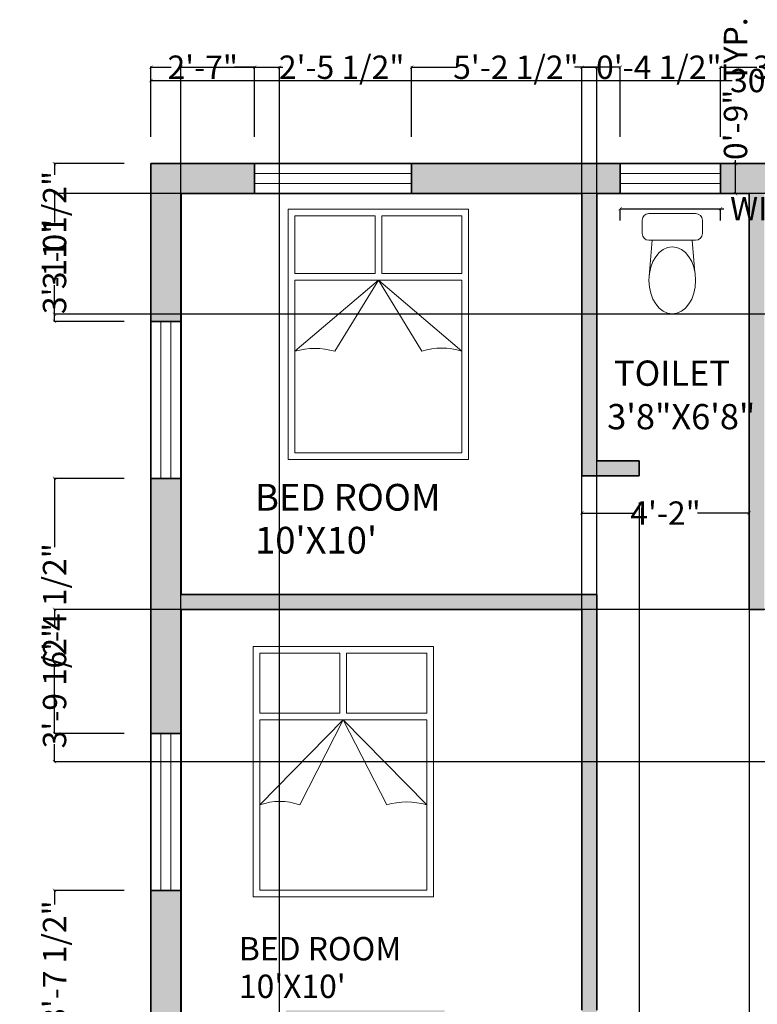
# Model space of a CAD drawing. Units: inches. Extents: x 98 to 545, y 56 to 703.
# Tile 3 of 4: x 103 to 324, y 408 to 703. Entities that reach past the tile are written whole.
import ezdxf

# ---------------------------------------------------------------- set-up
doc = ezdxf.new("R2010")
doc.units = ezdxf.units.IN
doc.header["$MEASUREMENT"] = 0
for name, color, linetype, lineweight in [('A-ANNO-DIMS', 2, 'Continuous', 18), ('A-AREA-IDEN', 7, 'Continuous', 25), ('A-FLOR-FIXT', 9, 'Continuous', 15), ('A-GLAZ', 4, 'Continuous', 18), ('A-WALL', 7, 'Continuous', 35), ('Furniture', 7, 'Continuous', 15)]:
    doc.layers.add(name, color=color, linetype=linetype, lineweight=lineweight)
doc.layers.add('A-WALL-PATT', color=18, linetype='Continuous', lineweight=13, true_color=0x000000)
doc.styles.get("Standard").update_dxf_attribs({"font": 'arial.ttf'})
doc.dimstyles.get("Standard").update_dxf_attribs({"dimtxt": 7, "dimasz": 1, "dimexe": 0.183, "dimexo": 8, "dimgap": 0.09, "dimtad": 0, "dimdec": 4, "dimzin": 0, "dimdsep": 46, "dimlunit": 3, "dimtxsty": 'Standard', "dimblk": 'ARCHTICK', "dimcen": 0, "dimclrd": 253, "dimclre": 251, "dimadec": 0, "dimazin": 0, "dimtfac": 1, "dimtdec": 4, "dimtofl": 0, "dimtmove": 0, "dimatfit": 3, "dimfxl": 1, "dimtolj": 1, "dimtzin": 0, "dimarcsym": 0})

# ---------------------------------------------------------------- blocks, each defined once
blk = doc.blocks.new('_ArchTick')
at = {"color": 0, "linetype": 'ByBlock', "const_width": 0.15}
blk.add_lwpolyline([(-0.5, -0.5), (0.5, 0.5)], dxfattribs=at)
blk = doc.blocks.new('*D4')
at = {"layer": 'A-ANNO-DIMS', "color": 0, "lineweight": -2, "transparency": 16777216}
for p, q in [((142.36, 667.7), (142.36, 684.75)), ((142.36, 684.57), (316.34, 684.57)), ((502.36, 684.57), (328.39, 684.57)), ((502.36, 667.7), (502.36, 684.75))]:
    blk.add_line(p, q, dxfattribs=at)
at = {"layer": 'Defpoints', "color": 0, "transparency": 16777216}
for p in [(502.36, 684.57), (142.36, 659.7), (502.36, 659.7)]:
    blk.add_point(p, dxfattribs=at)
at = {"layer": 'A-ANNO-DIMS', "color": 0, "lineweight": -2, "transparency": 16777216, "rotation": 180}
blk.add_blockref('_ArchTick', (142.36, 684.57), dxfattribs=at)
at = {"layer": 'A-ANNO-DIMS', "color": 0, "lineweight": -2, "transparency": 16777216}
blk.add_blockref('_ArchTick', (502.36, 684.57), dxfattribs=at)
at = {"layer": 'A-ANNO-DIMS', "color": 0, "transparency": 16777216, "insert": (322.36, 684.57), "char_height": 7, "attachment_point": 5}
blk.add_mtext("\\A1;30'", dxfattribs=at)
blk = doc.blocks.new('WIN-SASH-47IN')
for p, q in [((47, 9), (0, 9)), ((0, 6), (47, 6)), ((0, 3), (47, 3)), ((0, 0), (47, 0))]:
    blk.add_line(p, q)
blk = doc.blocks.new('WIN-SASH-30IN')
for p, q in [((30, 9), (0, 9)), ((0, 6), (30, 6)), ((0, 3), (30, 3)), ((0, 0), (30, 0))]:
    blk.add_line(p, q)
blk = doc.blocks.new('*D13')
at = {"layer": 'A-ANNO-DIMS', "color": 253, "lineweight": -2, "transparency": 16777216}
for p, q in [((282.86, 646.2), (312.86, 646.2)), ((312.86, 646.2), (313.86, 646.2))]:
    blk.add_line(p, q, dxfattribs=at)
at = {"layer": 'A-ANNO-DIMS', "color": 251, "lineweight": -2, "transparency": 16777216}
for p, q in [((282.86, 642.7), (282.86, 646.01)), ((312.86, 642.7), (312.86, 646.01))]:
    blk.add_line(p, q, dxfattribs=at)
at = {"layer": 'Defpoints', "color": 0, "transparency": 16777216}
for p in [(282.86, 650.7), (312.86, 650.7), (312.86, 646.2)]:
    blk.add_point(p, dxfattribs=at)
at = {"layer": 'A-ANNO-DIMS', "color": 253, "lineweight": -2, "transparency": 16777216, "rotation": 180}
blk.add_blockref('_ArchTick', (282.86, 646.2), dxfattribs=at)
at = {"layer": 'A-ANNO-DIMS', "color": 253, "lineweight": -2, "transparency": 16777216}
blk.add_blockref('_ArchTick', (312.86, 646.2), dxfattribs=at)
at = {"layer": 'A-ANNO-DIMS', "color": 0, "transparency": 16777216, "insert": (358.24, 646.2), "char_height": 7, "attachment_point": 5}
blk.add_mtext('\\A1;WINDOW 2\'-6" TYP.', dxfattribs=at)
blk = doc.blocks.new('*D14')
at = {"layer": 'A-ANNO-DIMS', "color": 253, "lineweight": -2, "transparency": 16777216}
for p, q in [((317.36, 659.7), (317.36, 660.7)), ((317.36, 650.7), (317.36, 659.7))]:
    blk.add_line(p, q, dxfattribs=at)
at = {"layer": 'A-ANNO-DIMS', "color": 251, "lineweight": -2, "transparency": 16777216}
for p, q in [((320.86, 659.7), (317.55, 659.7)), ((320.86, 650.7), (317.55, 650.7))]:
    blk.add_line(p, q, dxfattribs=at)
at = {"layer": 'Defpoints', "color": 0, "transparency": 16777216}
for p in [(312.86, 659.7), (317.36, 659.7), (312.86, 650.7)]:
    blk.add_point(p, dxfattribs=at)
at = {"layer": 'A-ANNO-DIMS', "color": 253, "lineweight": -2, "transparency": 16777216}
for p, rotation in [((317.36, 659.7), 90), ((317.36, 650.7), 270)]:
    blk.add_blockref('_ArchTick', p, dxfattribs=dict(at, rotation=rotation))
at = {"layer": 'A-ANNO-DIMS', "color": 0, "transparency": 16777216, "insert": (317.36, 682.12), "char_height": 7, "attachment_point": 5, "rotation": 90}
blk.add_mtext('\\A1;0\'-9" TYP.', dxfattribs=at)
blk = doc.blocks.new('*D21')
at = {"layer": 'A-ANNO-DIMS', "color": 251, "lineweight": -2, "transparency": 16777216}
for p, q in [((142.36, 667.7), (142.36, 688.73)), ((173.4, 667.7), (173.4, 688.73))]:
    blk.add_line(p, q, dxfattribs=at)
at = {"layer": 'A-ANNO-DIMS', "color": 253, "lineweight": -2, "transparency": 16777216}
for p, q in [((142.36, 688.55), (148.43, 688.55)), ((173.4, 688.55), (167.33, 688.55))]:
    blk.add_line(p, q, dxfattribs=at)
at = {"layer": 'Defpoints', "color": 0, "transparency": 16777216}
for p in [(173.4, 688.55), (142.36, 659.7), (173.4, 659.7)]:
    blk.add_point(p, dxfattribs=at)
at = {"layer": 'A-ANNO-DIMS', "color": 253, "lineweight": -2, "transparency": 16777216, "rotation": 180}
blk.add_blockref('_ArchTick', (142.36, 688.55), dxfattribs=at)
at = {"layer": 'A-ANNO-DIMS', "color": 253, "lineweight": -2, "transparency": 16777216}
blk.add_blockref('_ArchTick', (173.4, 688.55), dxfattribs=at)
at = {"layer": 'A-ANNO-DIMS', "color": 0, "transparency": 16777216, "insert": (157.88, 688.55), "char_height": 7, "attachment_point": 5}
blk.add_mtext('\\A1;2\'-7"', dxfattribs=at)
blk = doc.blocks.new('*D22')
at = {"layer": 'A-ANNO-DIMS', "color": 251, "lineweight": -2, "transparency": 16777216}
for p, q in [((220.4, 667.7), (220.4, 688.73)), ((282.86, 667.7), (282.86, 688.73))]:
    blk.add_line(p, q, dxfattribs=at)
at = {"layer": 'A-ANNO-DIMS', "color": 253, "lineweight": -2, "transparency": 16777216}
for p, q in [((220.4, 688.55), (234.08, 688.55)), ((282.86, 688.55), (269.18, 688.55))]:
    blk.add_line(p, q, dxfattribs=at)
at = {"layer": 'Defpoints', "color": 0, "transparency": 16777216}
for p in [(282.86, 688.55), (220.4, 659.7), (282.86, 659.7)]:
    blk.add_point(p, dxfattribs=at)
at = {"layer": 'A-ANNO-DIMS', "color": 253, "lineweight": -2, "transparency": 16777216, "rotation": 180}
blk.add_blockref('_ArchTick', (220.4, 688.55), dxfattribs=at)
at = {"layer": 'A-ANNO-DIMS', "color": 253, "lineweight": -2, "transparency": 16777216}
blk.add_blockref('_ArchTick', (282.86, 688.55), dxfattribs=at)
at = {"layer": 'A-ANNO-DIMS', "color": 0, "transparency": 16777216, "insert": (251.63, 688.55), "char_height": 7, "attachment_point": 5}
blk.add_mtext('\\A1;5\'-2 1/2"', dxfattribs=at)
blk = doc.blocks.new('*D23')
at = {"layer": 'A-ANNO-DIMS', "color": 251, "lineweight": -2, "transparency": 16777216}
for p, q in [((312.86, 667.7), (312.86, 688.73)), ((358.82, 667.7), (358.82, 688.73))]:
    blk.add_line(p, q, dxfattribs=at)
at = {"layer": 'A-ANNO-DIMS', "color": 253, "lineweight": -2, "transparency": 16777216}
for p, q in [((312.86, 688.55), (323.73, 688.55)), ((358.82, 688.55), (347.95, 688.55))]:
    blk.add_line(p, q, dxfattribs=at)
at = {"layer": 'Defpoints', "color": 0, "transparency": 16777216}
for p in [(358.82, 688.55), (312.86, 659.7), (358.82, 659.7)]:
    blk.add_point(p, dxfattribs=at)
at = {"layer": 'A-ANNO-DIMS', "color": 253, "lineweight": -2, "transparency": 16777216, "rotation": 180}
blk.add_blockref('_ArchTick', (312.86, 688.55), dxfattribs=at)
at = {"layer": 'A-ANNO-DIMS', "color": 253, "lineweight": -2, "transparency": 16777216}
blk.add_blockref('_ArchTick', (358.82, 688.55), dxfattribs=at)
at = {"layer": 'A-ANNO-DIMS', "color": 0, "transparency": 16777216, "insert": (335.84, 688.55), "char_height": 7, "attachment_point": 5}
blk.add_mtext('\\A1;3\'-10"', dxfattribs=at)
blk = doc.blocks.new('*D25')
at = {"layer": 'A-ANNO-DIMS', "color": 251, "lineweight": -2, "transparency": 16777216}
for p, q in [((134.36, 659.7), (113.33, 659.7)), ((134.36, 612.44), (113.33, 612.44))]:
    blk.add_line(p, q, dxfattribs=at)
at = {"layer": 'A-ANNO-DIMS', "color": 253, "lineweight": -2, "transparency": 16777216}
for p, q in [((113.51, 659.7), (113.51, 656.34)), ((113.51, 612.44), (113.51, 615.8))]:
    blk.add_line(p, q, dxfattribs=at)
at = {"layer": 'Defpoints', "color": 0, "transparency": 16777216}
for p in [(142.36, 659.7), (113.51, 612.44), (142.36, 612.44)]:
    blk.add_point(p, dxfattribs=at)
at = {"layer": 'A-ANNO-DIMS', "color": 253, "lineweight": -2, "transparency": 16777216}
for p, rotation in [((113.51, 659.7), 90), ((113.51, 612.44), 270)]:
    blk.add_blockref('_ArchTick', p, dxfattribs=dict(at, rotation=rotation))
at = {"layer": 'A-ANNO-DIMS', "color": 0, "transparency": 16777216, "insert": (113.51, 636.07), "char_height": 7, "attachment_point": 5, "rotation": 90}
blk.add_mtext('\\A1;3\'-11 1/2"', dxfattribs=at)
blk = doc.blocks.new('*D26')
at = {"layer": 'A-ANNO-DIMS', "color": 251, "lineweight": -2, "transparency": 16777216}
for p, q in [((134.36, 565.44), (113.33, 565.44)), ((134.36, 489.08), (113.33, 489.08))]:
    blk.add_line(p, q, dxfattribs=at)
at = {"layer": 'A-ANNO-DIMS', "color": 253, "lineweight": -2, "transparency": 16777216}
for p, q in [((113.51, 565.44), (113.51, 544.83)), ((113.51, 489.08), (113.51, 509.69))]:
    blk.add_line(p, q, dxfattribs=at)
at = {"layer": 'Defpoints', "color": 0, "transparency": 16777216}
for p in [(142.36, 565.44), (113.51, 489.08), (142.36, 489.08)]:
    blk.add_point(p, dxfattribs=at)
at = {"layer": 'A-ANNO-DIMS', "color": 253, "lineweight": -2, "transparency": 16777216}
for p, rotation in [((113.51, 565.44), 90), ((113.51, 489.08), 270)]:
    blk.add_blockref('_ArchTick', p, dxfattribs=dict(at, rotation=rotation))
at = {"layer": 'A-ANNO-DIMS', "color": 0, "transparency": 16777216, "insert": (113.51, 527.26), "char_height": 7, "attachment_point": 5, "rotation": 90}
blk.add_mtext('\\A1;6\'-4 1/2"', dxfattribs=at)
blk = doc.blocks.new('*D27')
at = {"layer": 'A-ANNO-DIMS', "color": 251, "lineweight": -2, "transparency": 16777216}
for p, q in [((134.36, 442.08), (113.33, 442.08)), ((134.36, 398.55), (113.33, 398.55))]:
    blk.add_line(p, q, dxfattribs=at)
at = {"layer": 'A-ANNO-DIMS', "color": 253, "lineweight": -2, "transparency": 16777216}
for p, q in [((113.51, 442.08), (113.51, 437.86)), ((113.51, 398.55), (113.51, 402.77))]:
    blk.add_line(p, q, dxfattribs=at)
at = {"layer": 'Defpoints', "color": 0, "transparency": 16777216}
for p in [(142.36, 442.08), (113.51, 398.55), (142.36, 398.55)]:
    blk.add_point(p, dxfattribs=at)
at = {"layer": 'A-ANNO-DIMS', "color": 253, "lineweight": -2, "transparency": 16777216}
for p, rotation in [((113.51, 442.08), 90), ((113.51, 398.55), 270)]:
    blk.add_blockref('_ArchTick', p, dxfattribs=dict(at, rotation=rotation))
at = {"layer": 'A-ANNO-DIMS', "color": 0, "transparency": 16777216, "insert": (113.51, 420.32), "char_height": 7, "attachment_point": 5, "rotation": 90}
blk.add_mtext('\\A1;3\'-7 1/2"', dxfattribs=at)
blk = doc.blocks.new('*D31')
at = {"layer": 'A-ANNO-DIMS', "color": 251, "lineweight": -2, "transparency": 16777216}
for p, q in [((485.36, 650.7), (113.33, 650.7)), ((485.36, 614.58), (113.33, 614.58))]:
    blk.add_line(p, q, dxfattribs=at)
at = {"layer": 'A-ANNO-DIMS', "color": 253, "lineweight": -2, "transparency": 16777216}
for p, q in [((113.51, 650.7), (113.51, 642.03)), ((113.51, 614.58), (113.51, 623.25))]:
    blk.add_line(p, q, dxfattribs=at)
at = {"layer": 'Defpoints', "color": 0, "transparency": 16777216}
for p in [(493.36, 650.7), (113.51, 614.58), (493.36, 614.58)]:
    blk.add_point(p, dxfattribs=at)
at = {"layer": 'A-ANNO-DIMS', "color": 253, "lineweight": -2, "transparency": 16777216}
for p, rotation in [((113.51, 650.7), 90), ((113.51, 614.58), 270)]:
    blk.add_blockref('_ArchTick', p, dxfattribs=dict(at, rotation=rotation))
at = {"layer": 'A-ANNO-DIMS', "color": 0, "transparency": 16777216, "insert": (113.51, 632.64), "char_height": 7, "attachment_point": 5, "rotation": 90}
blk.add_mtext('\\A1;3\'-0"', dxfattribs=at)
blk = doc.blocks.new('*D32')
at = {"layer": 'A-ANNO-DIMS', "color": 251, "lineweight": -2, "transparency": 16777216}
for p, q in [((485.36, 526.2), (113.33, 526.2)), ((485.36, 480.62), (113.33, 480.62))]:
    blk.add_line(p, q, dxfattribs=at)
at = {"layer": 'A-ANNO-DIMS', "color": 253, "lineweight": -2, "transparency": 16777216}
for p, q in [((113.51, 526.2), (113.51, 520.96)), ((113.51, 480.62), (113.51, 485.86))]:
    blk.add_line(p, q, dxfattribs=at)
at = {"layer": 'Defpoints', "color": 0, "transparency": 16777216}
for p in [(493.36, 526.2), (113.51, 480.62), (493.36, 480.62)]:
    blk.add_point(p, dxfattribs=at)
at = {"layer": 'A-ANNO-DIMS', "color": 253, "lineweight": -2, "transparency": 16777216}
for p, rotation in [((113.51, 526.2), 90), ((113.51, 480.62), 270)]:
    blk.add_blockref('_ArchTick', p, dxfattribs=dict(at, rotation=rotation))
at = {"layer": 'A-ANNO-DIMS', "color": 0, "transparency": 16777216, "insert": (113.51, 503.41), "char_height": 7, "attachment_point": 5, "rotation": 90}
blk.add_mtext('\\A1;3\'-9 1/2"', dxfattribs=at)
blk = doc.blocks.new('*D41')
at = {"layer": 'A-ANNO-DIMS', "color": 251, "lineweight": -2, "transparency": 16777216}
for p, q in [((151.36, 314.3), (151.36, 688.73)), ((180.85, 314.3), (180.85, 688.73))]:
    blk.add_line(p, q, dxfattribs=at)
at = {"layer": 'A-ANNO-DIMS', "color": 253, "lineweight": -2, "transparency": 16777216}
for p, q in [((151.36, 688.55), (180.85, 688.55)), ((180.85, 688.55), (181.85, 688.55))]:
    blk.add_line(p, q, dxfattribs=at)
at = {"layer": 'Defpoints', "color": 0, "transparency": 16777216}
for p in [(180.85, 688.55), (151.36, 306.3), (180.85, 306.3)]:
    blk.add_point(p, dxfattribs=at)
at = {"layer": 'A-ANNO-DIMS', "color": 253, "lineweight": -2, "transparency": 16777216, "rotation": 180}
blk.add_blockref('_ArchTick', (151.36, 688.55), dxfattribs=at)
at = {"layer": 'A-ANNO-DIMS', "color": 253, "lineweight": -2, "transparency": 16777216}
blk.add_blockref('_ArchTick', (180.85, 688.55), dxfattribs=at)
at = {"layer": 'A-ANNO-DIMS', "color": 0, "transparency": 16777216, "insert": (199.46, 688.55), "char_height": 7, "attachment_point": 5}
blk.add_mtext('\\A1;2\'-5 1/2"', dxfattribs=at)
blk = doc.blocks.new('*D42')
at = {"layer": 'A-ANNO-DIMS', "color": 251, "lineweight": -2, "transparency": 16777216}
for p, q in [((288.56, 558.2), (288.56, 66.66)), ((321.46, 558.2), (321.46, 66.66))]:
    blk.add_line(p, q, dxfattribs=at)
at = {"layer": 'A-ANNO-DIMS', "color": 253, "lineweight": -2, "transparency": 16777216}
for p, q in [((288.56, 66.85), (295.56, 66.85)), ((321.46, 66.85), (314.46, 66.85))]:
    blk.add_line(p, q, dxfattribs=at)
at = {"layer": 'Defpoints', "color": 0, "transparency": 16777216}
for p in [(288.56, 566.2), (321.46, 566.2), (321.46, 66.85)]:
    blk.add_point(p, dxfattribs=at)
at = {"layer": 'A-ANNO-DIMS', "color": 253, "lineweight": -2, "transparency": 16777216, "rotation": 180}
blk.add_blockref('_ArchTick', (288.56, 66.85), dxfattribs=at)
at = {"layer": 'A-ANNO-DIMS', "color": 253, "lineweight": -2, "transparency": 16777216}
blk.add_blockref('_ArchTick', (321.46, 66.85), dxfattribs=at)
at = {"layer": 'A-ANNO-DIMS', "color": 0, "transparency": 16777216, "insert": (305.01, 66.85), "char_height": 7, "attachment_point": 5}
blk.add_mtext('\\A1;2\'-9"', dxfattribs=at)
blk = doc.blocks.new('*D44')
at = {"layer": 'A-ANNO-DIMS', "color": 251, "lineweight": -2, "transparency": 16777216}
for p, q in [((271.36, 534.2), (271.36, 555.23)), ((321.46, 534.2), (321.46, 555.23))]:
    blk.add_line(p, q, dxfattribs=at)
at = {"layer": 'A-ANNO-DIMS', "color": 253, "lineweight": -2, "transparency": 16777216}
for p, q in [((271.36, 555.05), (286.88, 555.05)), ((321.46, 555.05), (305.95, 555.05))]:
    blk.add_line(p, q, dxfattribs=at)
at = {"layer": 'Defpoints', "color": 0, "transparency": 16777216}
for p in [(321.46, 555.05), (271.36, 526.2), (321.46, 526.2)]:
    blk.add_point(p, dxfattribs=at)
at = {"layer": 'A-ANNO-DIMS', "color": 253, "lineweight": -2, "transparency": 16777216, "rotation": 180}
blk.add_blockref('_ArchTick', (271.36, 555.05), dxfattribs=at)
at = {"layer": 'A-ANNO-DIMS', "color": 253, "lineweight": -2, "transparency": 16777216}
blk.add_blockref('_ArchTick', (321.46, 555.05), dxfattribs=at)
at = {"layer": 'A-ANNO-DIMS', "color": 0, "transparency": 16777216, "insert": (296.41, 555.05), "char_height": 7, "attachment_point": 5}
blk.add_mtext('\\A1;4\'-2"', dxfattribs=at)
blk = doc.blocks.new('*D47')
at = {"layer": 'A-ANNO-DIMS', "color": 251, "lineweight": -2, "transparency": 16777216}
for p, q in [((271.36, 409.7), (271.36, 688.73)), ((275.86, 409.7), (275.86, 688.73))]:
    blk.add_line(p, q, dxfattribs=at)
at = {"layer": 'A-ANNO-DIMS', "color": 253, "lineweight": -2, "transparency": 16777216}
for p, q in [((271.36, 688.55), (275.86, 688.55)), ((275.86, 688.55), (276.86, 688.55))]:
    blk.add_line(p, q, dxfattribs=at)
at = {"layer": 'Defpoints', "color": 0, "transparency": 16777216}
for p in [(275.86, 688.55), (271.36, 401.7), (275.86, 401.7)]:
    blk.add_point(p, dxfattribs=at)
at = {"layer": 'A-ANNO-DIMS', "color": 253, "lineweight": -2, "transparency": 16777216, "rotation": 180}
blk.add_blockref('_ArchTick', (271.36, 688.55), dxfattribs=at)
at = {"layer": 'A-ANNO-DIMS', "color": 253, "lineweight": -2, "transparency": 16777216}
blk.add_blockref('_ArchTick', (275.86, 688.55), dxfattribs=at)
at = {"layer": 'A-ANNO-DIMS', "color": 0, "transparency": 16777216, "insert": (294.41, 688.55), "char_height": 7, "attachment_point": 5}
blk.add_mtext('\\A1;0\'-4 1/2"', dxfattribs=at)

msp = doc.modelspace()

# ---------------------------------------------------------------- hatches: boundary and pattern name
at = {"layer": 'A-WALL-PATT'}
h = msp.add_hatch(color=256, dxfattribs=at)
h.dxf.hatch_style = 1
h.paths.add_polyline_path([(173.39577, 659.69681), (142.36469, 659.69681), (142.36469, 612.44216), (151.36469, 612.44216), (151.36469, 650.69681), (173.39577, 650.69681)])
h.paths.add_polyline_path([(282.86266, 659.69681), (220.39577, 659.69681), (220.39577, 650.69681), (271.36469, 650.69681), (271.36469, 566.19681), (275.86469, 566.19681), (288.55623, 566.19681), (288.55623, 570.69681), (275.86469, 570.69681), (275.86469, 650.69681), (282.86266, 650.69681)])
h.paths.add_polyline_path([(358.82163, 659.69681), (312.86266, 659.69681), (312.86266, 650.69681), (321.46469, 650.69681), (321.46469, 570.69681), (321.46469, 566.19681), (321.46469, 530.69681), (321.46469, 526.19681), (325.96469, 526.19681), (325.96469, 530.69681), (325.96469, 650.69681), (358.82163, 650.69681)])
h.paths.add_polyline_path([(451.98971, 659.69681), (405.82163, 659.69681), (405.82163, 650.69681), (435.16469, 650.69681), (435.16469, 570.08746), (439.66469, 570.08746), (439.66469, 650.69681), (451.98971, 650.69681)])
h.paths.add_polyline_path([(502.36469, 659.69681), (481.98971, 659.69681), (481.98971, 650.69681), (493.36469, 650.69681), (493.36469, 614.57752), (502.36469, 614.57752)])
h.paths.add_polyline_path([(502.36469, 579.57752), (493.36469, 579.57752), (493.36469, 530.69681), (439.66469, 530.69681), (435.16469, 530.69681), (373.81242, 530.69681), (373.81242, 526.19681), (493.36469, 526.19681), (493.36469, 480.62471), (502.36469, 480.62471)])
h.paths.add_polyline_path([(502.36469, 445.62471), (493.36469, 445.62471), (493.36469, 406.19681), (493.36469, 401.69681), (493.36469, 397.69681), (379.47742, 397.69681), (379.47742, 393.19681), (493.36469, 393.19681), (493.36469, 306.38501), (502.36469, 306.38501)])
h.paths.add_polyline_path([(502.36469, 271.38501), (493.36469, 271.38501), (493.36469, 193.19681), (478.76571, 193.19681), (478.76571, 188.69681), (493.36469, 188.69681), (493.36469, 128.69681), (487.75103, 128.69681), (487.75103, 119.69681), (502.36469, 119.69681)])
h.paths.add_polyline_path([(452.75103, 128.69681), (445.36469, 128.69681), (445.36469, 188.69681), (456.12508, 188.69681), (456.12508, 193.19681), (440.86469, 193.19681), (440.86469, 119.69681), (452.75103, 119.69681)])
h.paths.add_polyline_path([(307.21941, 128.69681), (293.86469, 128.69681), (293.86469, 188.69681), (404.74827, 188.69681), (404.74827, 193.19681), (293.86469, 193.19681), (293.86469, 306.29681), (289.36469, 306.29681), (289.36469, 119.69681), (307.21941, 119.69681)])
h.paths.add_polyline_path([(289.36469, 161.69681), (238.02122, 161.69681), (238.02122, 152.69681), (289.36469, 152.69681)])
h.paths.add_polyline_path([(191.02122, 161.69681), (151.36469, 161.69681), (151.36469, 191.65928), (142.36469, 191.65928), (142.36469, 152.69681), (151.36469, 152.69681), (191.02122, 152.69681)])
h.paths.add_polyline_path([(151.36469, 306.29681), (151.36469, 308.54862), (142.36469, 308.54862), (142.36469, 238.65928), (151.36469, 238.65928)])
h.paths.add_polyline_path([(230.26469, 401.69681), (230.26469, 406.19681), (182.81458, 406.19681), (182.81458, 401.69681), (225.76469, 401.69681), (225.76469, 358.49681), (151.36469, 358.49681), (151.36469, 368.55378), (142.36469, 368.55378), (142.36469, 338.54862), (151.36469, 338.54862), (151.36469, 353.99681), (225.76469, 353.99681), (225.76469, 310.79681), (180.84919, 310.79681), (180.84919, 306.29681), (230.26469, 306.29681)])
h.paths.add_polyline_path([(151.36469, 442.07867), (142.36469, 442.07867), (142.36469, 398.55378), (151.36469, 398.55378), (151.36469, 401.69681)])
h.paths.add_polyline_path([(151.36469, 526.19681), (271.36469, 526.19681), (271.36469, 406.19681), (271.36469, 401.69681), (275.86469, 401.69681), (275.86469, 406.19681), (275.86469, 526.19681), (275.86469, 530.69681), (271.36469, 530.69681), (151.36469, 530.69681), (151.36469, 565.44216), (142.36469, 565.44216), (142.36469, 489.07867), (151.36469, 489.07867)])

# ---------------------------------------------------------------- linework, layer by layer
at = {"layer": 'A-FLOR-FIXT'}
for p, q in [((289.43118, 638.74495), (289.43118, 642.74495)), ((291.43118, 644.74495), (305.43118, 644.74495)), ((307.43118, 642.74495), (307.43118, 638.74495)), ((305.43118, 636.74495), (291.43118, 636.74495)), ((292.43118, 636.74495), (291.48574, 625.9911)), ((304.43118, 636.74495), (305.22914, 627.13012))]:
    msp.add_line(p, q, dxfattribs=at)
for centre, start, end in [((291.43118, 642.74495), 90, 180), ((305.43118, 642.74495), 0, 90), ((291.43118, 638.74495), 180, 270), ((305.43118, 638.74495), 270, 0)]:
    msp.add_arc(centre, 2, start, end, dxfattribs=at)
msp.add_ellipse((298.43118, 624.74495), major_axis=(0, -10), ratio=0.7, dxfattribs=at)
at = {"layer": 'A-WALL'}
for p, q in [((502.36469, 659.69681), (142.36469, 659.69681)), ((142.36469, 659.69681), (142.36469, 152.69681)), ((173.39577, 659.69681), (173.39577, 650.69681)), ((220.39577, 650.69681), (220.39577, 659.69681)), ((282.86266, 659.69681), (282.86266, 650.69681)), ((312.86266, 650.69681), (312.86266, 659.69681)), ((151.36469, 650.69681), (151.36469, 530.69681)), ((271.36469, 650.69681), (151.36469, 650.69681)), ((271.36469, 650.69681), (271.36469, 566.19681)), ((275.86469, 650.69681), (275.86469, 570.69681)), ((321.46469, 650.69681), (275.86469, 650.69681)), ((321.46469, 650.69681), (321.46469, 570.69681)), ((142.36469, 612.44216), (151.36469, 612.44216)), ((288.55623, 570.69681), (275.86469, 570.69681)), ((288.55623, 570.69681), (288.55623, 566.19681)), ((321.46469, 566.19681), (321.46469, 570.69681)), ((275.86469, 566.19681), (271.36469, 566.19681)), ((288.55623, 566.19681), (275.86469, 566.19681)), ((321.46469, 566.19681), (321.46469, 530.69681)), ((151.36469, 565.44216), (142.36469, 565.44216)), ((271.36469, 530.69681), (151.36469, 530.69681)), ((275.86469, 530.69681), (271.36469, 530.69681)), ((275.86469, 526.19681), (275.86469, 530.69681)), ((321.46469, 530.69681), (321.46469, 526.19681)), ((151.36469, 526.19681), (151.36469, 401.69681)), ((271.36469, 526.19681), (151.36469, 526.19681)), ((271.36469, 526.19681), (271.36469, 406.19681)), ((275.86469, 526.19681), (275.86469, 406.19681)), ((325.96469, 526.19681), (321.46469, 526.19681)), ((142.36469, 489.07867), (151.36469, 489.07867)), ((151.36469, 442.07867), (142.36469, 442.07867))]:
    msp.add_line(p, q, dxfattribs=at)
at = {"layer": 'Furniture'}
for p, q in [((183.44555, 646.08207), (237.44555, 646.08207)), ((183.44555, 571.08207), (183.44555, 646.08207)), ((237.44555, 646.08207), (237.44555, 571.08207)), ((185.44555, 644.08207), (209.44555, 644.08207)), ((185.44555, 626.75259), (185.44555, 644.08207)), ((209.44555, 626.75259), (209.44555, 644.08207)), ((211.44555, 626.75259), (211.44555, 644.08207)), ((211.44555, 644.08207), (235.44555, 644.08207)), ((235.44555, 644.08207), (235.44555, 626.75259)), ((185.44555, 626.75259), (209.44555, 626.75259)), ((211.44555, 626.75259), (235.44555, 626.75259)), ((185.44555, 573.08207), (185.44555, 624.75259)), ((185.44555, 624.75259), (235.44555, 624.75259)), ((210.44555, 624.75259), (185.44555, 603.48914)), ((197.44555, 603.48914), (210.44555, 624.75259)), ((210.44555, 624.75259), (235.44555, 603.48914)), ((223.44555, 603.48914), (210.44555, 624.75259)), ((235.44555, 624.75259), (235.44555, 573.08207)), ((235.44555, 573.08207), (185.44555, 573.08207)), ((237.44555, 571.08207), (183.44555, 571.08207)), ((172.94351, 515.14937), (226.94351, 515.14937)), ((172.94351, 440.14937), (172.94351, 515.14937)), ((174.94351, 513.14937), (198.94351, 513.14937)), ((174.94351, 495.19226), (174.94351, 513.14937)), ((198.94351, 495.19226), (198.94351, 513.14937)), ((200.94351, 495.19226), (200.94351, 513.14937)), ((200.94351, 513.14937), (224.94351, 513.14937)), ((224.94351, 513.14937), (224.94351, 495.19226)), ((226.94351, 515.14937), (226.94351, 440.14937)), ((174.94351, 495.19226), (198.94351, 495.19226)), ((174.94351, 442.14937), (174.94351, 493.19226)), ((174.94351, 493.19226), (224.94351, 493.19226)), ((199.94351, 493.19226), (174.94351, 467.67082)), ((186.94351, 467.67082), (199.94351, 493.19226)), ((199.94351, 493.19226), (224.94351, 467.67082)), ((212.94351, 467.67082), (199.94351, 493.19226)), ((200.94351, 495.19226), (224.94351, 495.19226)), ((224.94351, 493.19226), (224.94351, 442.14937)), ((226.94351, 440.14937), (172.94351, 440.14937)), ((224.94351, 442.14937), (174.94351, 442.14937))]:
    msp.add_line(p, q, dxfattribs=at)
for centre, radius, start, end in [((229.44555, 585.79749), 18.68139, 71.2659893, 108.7340107), ((191.44555, 583.41307), 20.95348, 73.3605238, 106.6394762), ((180.94351, 450.92556), 17.78774, 70.2868714, 109.7131286), ((218.94351, 447.5256), 21.01975, 73.4144992, 106.5855008)]:
    msp.add_arc(centre, radius, start, end, dxfattribs=at)

# ---------------------------------------------------------------- block references
at = {"layer": 'A-GLAZ'}
for p, rotation in [((220.3954, 659.69661), 180), ((151.3645, 565.44253), 89.99999999999967), ((151.3645, 442.07904), 89.99999999999969)]:
    msp.add_blockref('WIN-SASH-47IN', p, dxfattribs=dict(at, rotation=rotation))
msp.add_blockref('WIN-SASH-30IN', (282.863, 650.697), dxfattribs=at)

# ---------------------------------------------------------------- texts
at = {"layer": 'A-AREA-IDEN'}
for s, p in [('TOILET', (280.98962, 593.16167)), ('3\'8"X6\'8"', (278.93954, 580.13813))]:
    msp.add_text(s, height=7.566418, rotation=0.0019444, dxfattribs=at).set_placement(p)
for s, height, p in [('BED ROOM', 8, (173.5144, 555.78549)), ("10'X10'     ", 8, (173.5144, 542.93419)), ('BED ROOM', 7, (168.68771, 421.10852)), ("10'X10'", 7, (168.68771, 409.86363))]:
    msp.add_text(s, height=height, dxfattribs=at).set_placement(p)

# ---------------------------------------------------------------- dimensions: what is measured, and where the dimension line sits
at = {"layer": 'A-ANNO-DIMS'}
dim = msp.add_linear_dim(base=(317.36266, 659.69681), p1=(312.86266, 650.69681), p2=(312.86266, 659.69681), angle=90, text='<> TYP.', dimstyle='Standard', override={"dimdec": 1, "dimlfac": 1, "dimrnd": 0, "dimzin": 1, "dimdsep": 46, "dimlunit": 4, "dimfrac": 2}, dxfattribs=at)
dim.commit()
dim.dimension.update_dxf_attribs({"geometry": '*D14', "text_midpoint": (317.36266, 682.12105)})
for base, p1, p2, override, picture, middle in [((180.84919, 688.54681), (151.36469, 306.29681), (180.84919, 306.29681), {"dimdec": 1, "dimlfac": 1, "dimrnd": 0, "dimzin": 1, "dimdsep": 46, "dimlunit": 4, "dimfrac": 2}, '*D41', (199.45829, 688.54681)), ((282.86266, 688.54681), (220.39577, 659.69681), (282.86266, 659.69681), {"dimdec": 1, "dimlfac": 1, "dimrnd": 0, "dimzin": 1, "dimdsep": 46, "dimlunit": 4, "dimfrac": 2}, '*D22', (251.62922, 688.54681)), ((275.86469, 688.54681), (271.36469, 401.69681), (275.86469, 401.69681), {"dimdec": 1, "dimlfac": 1, "dimrnd": 0, "dimzin": 1, "dimdsep": 46, "dimlunit": 4, "dimfrac": 2}, '*D47', (294.41411, 688.54681)), ((173.39577, 688.54681), (142.36469, 659.69681), (173.39577, 659.69681), {"dimdec": 1, "dimlfac": 1, "dimrnd": 0, "dimzin": 1, "dimdsep": 46, "dimlunit": 4, "dimfrac": 2}, '*D21', (157.88023, 688.54681)), ((358.82163, 688.54681), (312.86266, 659.69681), (358.82163, 659.69681), {"dimdec": 1, "dimlfac": 1, "dimrnd": 0, "dimzin": 1, "dimdsep": 46, "dimlunit": 4, "dimfrac": 2}, '*D23', (335.84215, 688.54681)), ((502.36469, 684.56988), (142.36469, 659.69681), (502.36469, 659.69681), {"dimclrd": 0, "dimclre": 0, "dimclrt": 0}, '*D4', (322.36469, 684.56988)), ((321.46469, 66.84681), (288.55623, 566.19681), (321.46469, 566.19681), {"dimdec": 1, "dimlfac": 1, "dimrnd": 0, "dimzin": 1, "dimdsep": 46, "dimlunit": 4, "dimfrac": 2}, '*D42', (305.01046, 66.84681)), ((321.46469, 555.04681), (271.36469, 526.19681), (321.46469, 526.19681), {"dimdec": 1, "dimlfac": 1, "dimrnd": 0, "dimzin": 1, "dimdsep": 46, "dimlunit": 4, "dimfrac": 2}, '*D44', (296.41469, 555.04681))]:
    dim = msp.add_linear_dim(base=base, p1=p1, p2=p2, dimstyle='Standard', override=override, dxfattribs=at)
    dim.commit()
    dim.dimension.update_dxf_attribs({"geometry": picture, "text_midpoint": middle})
dim = msp.add_linear_dim(base=(312.86266, 646.19681), p1=(282.86266, 650.69681), p2=(312.86266, 650.69681), text='WINDOW <> TYP.', dimstyle='Standard', override={"dimdec": 1, "dimlfac": 1, "dimrnd": 0, "dimzin": 1, "dimdsep": 46, "dimlunit": 4, "dimfrac": 2}, dxfattribs=at)
dim.commit()
dim.dimension.update_dxf_attribs({"geometry": '*D13', "text_midpoint": (358.24222, 646.19681)})
for base, p1, p2, picture, middle in [((113.51469, 612.44216), (142.36469, 659.69681), (142.36469, 612.44216), '*D25', (113.51469, 636.06948)), ((113.51469, 614.57752), (493.36469, 650.69681), (493.36469, 614.57752), '*D31', (113.51469, 632.63716)), ((113.51469, 489.07867), (142.36469, 565.44216), (142.36469, 489.07867), '*D26', (113.51469, 527.26041)), ((113.51469, 480.62471), (493.36469, 526.19681), (493.36469, 480.62471), '*D32', (113.51469, 503.41076)), ((113.51469, 398.55378), (142.36469, 442.07867), (142.36469, 398.55378), '*D27', (113.51469, 420.31622))]:
    dim = msp.add_linear_dim(base=base, p1=p1, p2=p2, angle=90, dimstyle='Standard', override={"dimdec": 1, "dimlfac": 1, "dimrnd": 0, "dimzin": 1, "dimdsep": 46, "dimlunit": 4, "dimfrac": 2}, dxfattribs=at)
    dim.commit()
    dim.dimension.update_dxf_attribs({"geometry": picture, "text_midpoint": middle})

doc.saveas('drawing.dxf')
